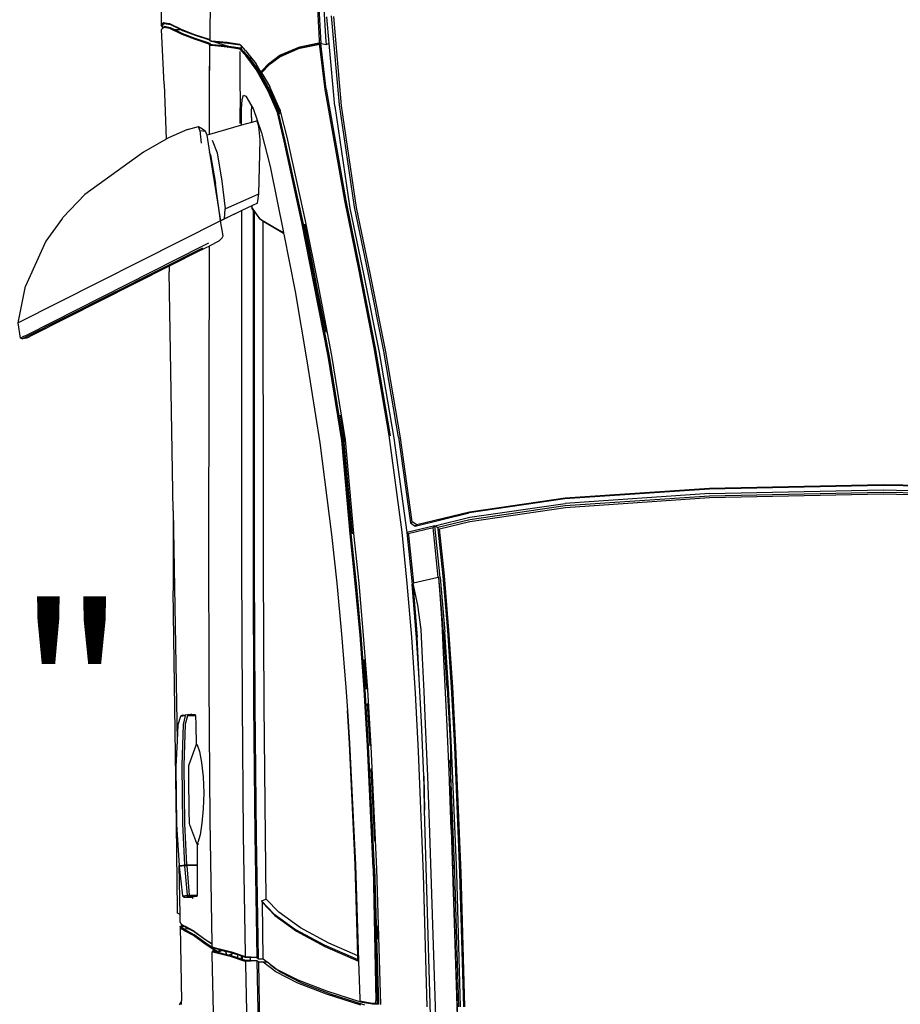
# Model space of a CAD drawing. Units: inches. Extents: x 0 to 4258, y 0 to 3769.
# Tile 10 of 30: x 3726 to 3761, y 3042 to 3082. Entities that reach past the tile are written whole.
import ezdxf

# ---------------------------------------------------------------- set-up
doc = ezdxf.new("R2010")
doc.units = ezdxf.units.IN
doc.header["$MEASUREMENT"] = 0
doc.layers.get('0').update_dxf_attribs({"color": 16})
doc.layers.add('A-ANNO-DIMS', color=250, linetype='Continuous', lineweight=18)
doc.layers.add('C-PKNG-VEHI', color=8, linetype='Continuous', lineweight=18)
doc.layers.add('Edges', color=250, linetype='Continuous')
doc.styles.get("Standard").update_dxf_attribs({"font": 'arial.ttf'})
doc.dimstyles.get("Standard").update_dxf_attribs({"dimtxt": 7, "dimasz": 0.18, "dimexe": 0.18, "dimexo": 0.0625, "dimgap": 0.09, "dimtad": 0, "dimtih": 1, "dimtoh": 1, "dimzin": 0, "dimdsep": 46, "dimlunit": 3, "dimtxsty": 'Standard', "dimcen": 0.09, "dimadec": 0, "dimazin": 0, "dimtfac": 1, "dimtofl": 0, "dimtmove": 0, "dimatfit": 3, "dimfxl": 1, "dimtolj": 1, "dimtzin": 0, "dimarcsym": 0})

# ---------------------------------------------------------------- blocks, each defined once
blk = doc.blocks.new('Nissan Qashqai pl')
at = {"layer": 'Edges'}
for p, q in [((9.2241, 12.1376), (9.2195, 11.9221)), ((9.2249, 12.1376), (9.2203, 11.9221)), ((9.2259, 11.9221), (9.2305, 12.1375)), ((9.2335, 12.1374), (9.2289, 11.9221)), ((9.2308, 11.9221), (9.2355, 12.1374)), ((9.2195, 11.9221), (9.2241, 11.7066)), ((9.2203, 11.9221), (9.2249, 11.7065)), ((9.2305, 11.7067), (9.2259, 11.9221)), ((9.2289, 11.9221), (9.2335, 11.7067)), ((9.2355, 11.7068), (9.2308, 11.9221)), ((9.2241, 11.7066), (9.2362, 11.5274)), ((9.2249, 11.7065), (9.2371, 11.5273)), ((9.2305, 11.7067), (9.2426, 11.5277)), ((9.2335, 11.7067), (9.2457, 11.5277)), ((9.2476, 11.5278), (9.2355, 11.7068)), ((9.2362, 11.5274), (9.2535, 11.4087)), ((9.2371, 11.5273), (9.2543, 11.4085)), ((9.2598, 11.4093), (9.2426, 11.5277)), ((9.2457, 11.5277), (9.2629, 11.4092)), ((9.2649, 11.4094), (9.2476, 11.5278)), ((9.2535, 11.4087), (9.2694, 11.3436)), ((9.2707, 11.3414), (9.2543, 11.4085)), ((9.2704, 11.3659), (9.2598, 11.4093)), ((9.2629, 11.4092), (9.2726, 11.3695)), ((9.2741, 11.3716), (9.2649, 11.4094)), ((9.8673, 11.4031), (9.701, 11.3983)), ((9.7011, 11.3963), (9.8673, 11.4012)), ((9.4706, 11.388), (9.4, 11.3832)), ((9.5443, 11.3919), (9.4706, 11.388)), ((9.4709, 11.3861), (9.5446, 11.39)), ((9.701, 11.3983), (9.5443, 11.3919)), ((9.5446, 11.39), (9.7011, 11.3963)), ((9.7014, 11.3929), (9.5454, 11.3866)), ((9.7014, 11.3906), (9.5695, 11.3853)), ((9.6472, 11.3861), (9.9278, 11.3949)), ((9.6714, 11.3874), (9.8565, 11.3931)), ((9.8673, 11.3977), (9.7014, 11.3929)), ((9.8673, 11.3954), (9.7014, 11.3906)), ((9.8565, 11.3931), (9.9794, 11.3967)), ((9.3326, 11.3776), (9.2741, 11.3716)), ((9.2746, 11.3697), (9.333, 11.3757)), ((9.4, 11.3832), (9.3326, 11.3776)), ((9.333, 11.3757), (9.4004, 11.3813)), ((9.4017, 11.3765), (9.3344, 11.3708)), ((9.3346, 11.3724), (9.4018, 11.378)), ((9.4276, 11.3767), (9.3918, 11.3747)), ((9.4004, 11.3813), (9.4709, 11.3861)), ((9.472, 11.3812), (9.4017, 11.3765)), ((9.472, 11.3828), (9.4018, 11.378)), ((9.4694, 11.3788), (9.4276, 11.3767)), ((9.5105, 11.3805), (9.4694, 11.3788)), ((9.5454, 11.3866), (9.472, 11.3828)), ((9.472, 11.3812), (9.5454, 11.3851)), ((9.5755, 11.3834), (9.5105, 11.3805)), ((9.5454, 11.3851), (9.5695, 11.3853)), ((9.5454, 11.3848), (9.5454, 11.3851)), ((9.5695, 11.3853), (9.5609, 11.3849)), ((9.5695, 11.3853), (9.5786, 11.3853)), ((9.6472, 11.3861), (9.5755, 11.3834)), ((9.5786, 11.3853), (9.6206, 11.3861)), ((9.6206, 11.3861), (9.6714, 11.3874)), ((9.3346, 11.3724), (9.2704, 11.3659)), ((9.2704, 11.3659), (9.2726, 11.3695)), ((9.2704, 11.3659), (9.2724, 11.3637)), ((9.2704, 11.3659), (9.2789, 11.331)), ((9.3346, 11.37), (9.2724, 11.3637)), ((9.2799, 11.3328), (9.2724, 11.3637)), ((9.2726, 11.3695), (9.2746, 11.3697)), ((9.3611, 11.3727), (9.3344, 11.3708)), ((9.3344, 11.3708), (9.3346, 11.37)), ((9.3346, 11.37), (9.3418, 11.3391)), ((9.3918, 11.3747), (9.3611, 11.3727)), ((9.6514, 11.3592), (9.9312, 11.3681)), ((9.4347, 11.3502), (9.4761, 11.3522)), ((9.4761, 11.3522), (9.5168, 11.3539)), ((9.5811, 11.3522), (9.514, 11.3492)), ((9.5168, 11.3539), (9.5812, 11.3568)), ((9.7029, 11.3516), (9.5503, 11.3455)), ((9.5811, 11.3522), (9.6231, 11.3531)), ((9.594, 11.3527), (9.5811, 11.3522)), ((9.5812, 11.3568), (9.6514, 11.3592)), ((9.6231, 11.3531), (9.594, 11.3527)), ((9.651, 11.3536), (9.6231, 11.3531)), ((9.9583, 11.363), (9.651, 11.3536)), ((9.8673, 11.3563), (9.7029, 11.3516)), ((9.2694, 11.3436), (9.2656, 11.3376)), ((9.2669, 11.3354), (9.2707, 11.3414)), ((9.2694, 11.3436), (9.2707, 11.3414)), ((9.2819, 11.333), (9.3418, 11.3391)), ((9.3418, 11.3391), (9.342, 11.3383)), ((9.342, 11.3383), (9.3687, 11.3441)), ((9.342, 11.3383), (9.4087, 11.3438)), ((9.4093, 11.3431), (9.3427, 11.3375)), ((9.3687, 11.3441), (9.3992, 11.3482)), ((9.3992, 11.3482), (9.4347, 11.3502)), ((9.4605, 11.3465), (9.4087, 11.3438)), ((9.4782, 11.3418), (9.4088, 11.3371)), ((9.4605, 11.3465), (9.4093, 11.3431)), ((9.514, 11.3492), (9.4605, 11.3465)), ((9.5503, 11.3455), (9.4782, 11.3418)), ((9.1605, 11.3208), (9.2669, 11.3354)), ((9.2656, 11.3376), (9.1612, 11.3233)), ((9.1617, 11.315), (9.2789, 11.331)), ((9.2669, 11.3354), (9.2656, 11.3376)), ((9.3422, 11.3316), (9.2783, 11.3251)), ((9.2789, 11.331), (9.3427, 11.3375)), ((9.2789, 11.331), (9.2799, 11.3327)), ((9.2799, 11.3328), (9.2819, 11.333)), ((9.2799, 11.3327), (9.2799, 11.3328)), ((9.2799, 11.3327), (9.2811, 11.3325)), ((9.4088, 11.3371), (9.3422, 11.3316)), ((9.1605, 11.3208), (9.0538, 11.3023)), ((9.1612, 11.3233), (9.0546, 11.3048)), ((9.0552, 11.2965), (9.1617, 11.315)), ((9.2783, 11.3251), (9.1584, 11.3091)), ((9.0538, 11.3023), (8.9583, 11.2833)), ((9.0546, 11.3048), (8.9591, 11.2859)), ((9.1584, 11.3091), (9.0495, 11.2906)), ((9.0497, 11.2918), (9.1586, 11.3104)), ((9.0495, 11.2906), (8.9521, 11.2715)), ((8.9522, 11.2728), (9.0497, 11.2918)), ((8.9598, 11.2775), (9.0552, 11.2965)), ((9.6954, 11.2907), (9.5438, 11.2836)), ((9.5443, 11.2863), (9.696, 11.2932)), ((9.5717, 11.2865), (9.6618, 11.2907)), ((9.6953, 11.2892), (9.863, 11.2944)), ((9.6953, 11.2892), (9.8598, 11.2925)), ((9.6954, 11.2907), (9.8641, 11.2959)), ((9.696, 11.2932), (9.8644, 11.2982)), ((9.7669, 11.2945), (9.7832, 11.2951)), ((9.8629, 11.2925), (9.8598, 11.2925)), ((9.8626, 11.2878), (9.8627, 11.2909)), ((9.8627, 11.2909), (9.8629, 11.2925)), ((9.8627, 11.2909), (9.8637, 11.291)), ((9.8629, 11.2925), (9.863, 11.2944)), ((9.8641, 11.2959), (9.863, 11.2944)), ((9.8635, 11.2886), (9.8637, 11.291)), ((9.8637, 11.291), (9.8638, 11.2934)), ((9.8637, 11.291), (9.8643, 11.291)), ((9.8638, 11.2934), (9.8641, 11.2959)), ((8.9583, 11.2833), (8.8745, 11.266)), ((8.9591, 11.2859), (8.8754, 11.2687)), ((8.8761, 11.2602), (8.9598, 11.2775)), ((9.4735, 11.2779), (9.4062, 11.2729)), ((9.4736, 11.2793), (9.4063, 11.2743)), ((9.4064, 11.277), (9.4739, 11.282)), ((9.4727, 11.2808), (9.4362, 11.278)), ((9.4727, 11.2808), (9.4732, 11.2808)), ((9.5437, 11.2822), (9.4735, 11.2779)), ((9.5438, 11.2836), (9.4736, 11.2793)), ((9.4739, 11.282), (9.5443, 11.2863)), ((9.491, 11.2819), (9.5434, 11.2852)), ((9.6953, 11.2892), (9.5437, 11.2822)), ((9.8652, 11.2788), (9.8516, 11.2363)), ((9.8605, 11.2746), (9.8626, 11.2878)), ((9.8615, 11.2754), (9.8635, 11.2886)), ((8.8745, 11.266), (8.7481, 11.2473)), ((8.8754, 11.2687), (8.7491, 11.2501)), ((8.8666, 11.2554), (8.9522, 11.2728)), ((8.9521, 11.2715), (8.8666, 11.2541)), ((9.2801, 11.2648), (9.3418, 11.2713)), ((9.3418, 11.2671), (9.2803, 11.2606)), ((9.3419, 11.2685), (9.2804, 11.262)), ((9.3418, 11.2713), (9.4064, 11.277)), ((9.4062, 11.2729), (9.3418, 11.2671)), ((9.4063, 11.2743), (9.3419, 11.2685)), ((9.5403, 11.26), (9.6913, 11.2674)), ((9.6912, 11.2667), (9.5404, 11.2598)), ((9.8039, 11.27), (9.6912, 11.2667)), ((9.6913, 11.2674), (9.8099, 11.2711)), ((9.8039, 11.27), (9.7884, 11.2343)), ((9.7905, 11.2283), (9.8087, 11.2702)), ((9.7925, 11.2294), (9.8107, 11.2711)), ((9.8087, 11.2702), (9.8039, 11.27)), ((9.8099, 11.2711), (9.8087, 11.2702)), ((9.8099, 11.2711), (9.8107, 11.2711)), ((9.8107, 11.2711), (9.8573, 11.2726)), ((9.8475, 11.2312), (9.8611, 11.2734)), ((9.8652, 11.2738), (9.8516, 11.2313)), ((9.8573, 11.2726), (9.8603, 11.2727)), ((9.8603, 11.2727), (9.8605, 11.2746)), ((9.8611, 11.2734), (9.8603, 11.2727)), ((9.8612, 11.2735), (9.8611, 11.2734)), ((9.8612, 11.2735), (9.8615, 11.2754)), ((8.7287, 11.2307), (8.8666, 11.2554)), ((8.8666, 11.2541), (8.7292, 11.2295)), ((8.7496, 11.2416), (8.8761, 11.2602)), ((9.0591, 11.2377), (9.1639, 11.2546)), ((9.133, 11.2481), (9.1647, 11.2532)), ((9.1639, 11.2546), (9.2801, 11.2648)), ((9.2803, 11.2606), (9.1644, 11.2503)), ((9.2804, 11.262), (9.1645, 11.2518)), ((9.1647, 11.2532), (9.1668, 11.2533)), ((9.2804, 11.2635), (9.1668, 11.2533)), ((9.4048, 11.2501), (9.471, 11.2554)), ((9.471, 11.2554), (9.4997, 11.2573)), ((9.4997, 11.2573), (9.5403, 11.26)), ((9.5404, 11.2598), (9.4997, 11.2573)), ((8.7481, 11.2473), (8.6375, 11.2376)), ((8.7491, 11.2501), (8.6386, 11.2404)), ((8.7496, 11.2416), (8.6721, 11.2348)), ((9.1644, 11.2503), (9.06, 11.2335)), ((9.1645, 11.2518), (9.0601, 11.235)), ((9.2814, 11.2377), (9.3416, 11.2442)), ((9.3416, 11.2442), (9.4048, 11.2501)), ((8.6699, 11.231), (8.622, 11.228)), ((8.6721, 11.2348), (8.6387, 11.2319)), ((8.6721, 11.2312), (8.6699, 11.231)), ((8.6721, 11.2348), (8.6733, 11.2313)), ((8.6721, 11.2312), (8.6721, 11.2318)), ((8.6721, 11.2241), (8.6733, 11.2313)), ((8.6733, 11.2313), (8.6721, 11.2312)), ((8.7287, 11.2307), (8.6721, 11.2241)), ((8.7292, 11.2295), (8.6753, 11.2232)), ((9.0601, 11.235), (8.8941, 11.2023)), ((8.9679, 11.2201), (9.0591, 11.2377)), ((9.06, 11.2335), (8.9696, 11.2157)), ((8.9708, 11.2185), (9.03, 11.2304)), ((9.1676, 11.2229), (9.2814, 11.2377)), ((9.7884, 11.2343), (9.7692, 11.1989)), ((9.7733, 11.194), (9.7925, 11.2294)), ((9.8338, 11.1956), (9.8475, 11.2312)), ((9.8516, 11.2363), (9.8378, 11.2007)), ((9.8516, 11.2313), (9.8378, 11.1957)), ((8.6683, 11.2226), (8.6197, 11.2201)), ((8.6203, 11.2213), (8.6721, 11.2241)), ((8.671, 11.2227), (8.6683, 11.2226)), ((8.6721, 11.2241), (8.671, 11.2227)), ((8.6716, 11.2199), (8.671, 11.2227)), ((8.6759, 11.1982), (8.6716, 11.2199)), ((8.6721, 11.2241), (8.6727, 11.2229)), ((8.6772, 11.1988), (8.6721, 11.2241)), ((8.6753, 11.2232), (8.6727, 11.2229)), ((8.6777, 11.1984), (8.6727, 11.2229)), ((8.8918, 11.205), (8.9679, 11.2201)), ((8.9318, 11.211), (8.9704, 11.2185)), ((8.9704, 11.2185), (8.9708, 11.2185)), ((9.0656, 11.207), (9.1676, 11.2229)), ((9.7713, 11.1929), (9.7905, 11.2283)), ((8.7881, 11.1821), (8.8918, 11.205)), ((8.9696, 11.2157), (8.8942, 11.2009)), ((8.8961, 11.204), (8.9318, 11.211)), ((8.9797, 11.1924), (9.0656, 11.207)), ((8.6864, 11.1736), (8.6759, 11.1982)), ((8.6875, 11.1744), (8.6772, 11.1988)), ((8.6777, 11.1984), (8.6883, 11.1737)), ((8.8941, 11.2023), (8.7925, 11.1802)), ((8.8942, 11.2009), (8.7931, 11.1789)), ((8.9087, 11.1783), (8.9797, 11.1924)), ((9.7692, 11.1989), (9.7499, 11.1721)), ((9.7519, 11.1661), (9.7713, 11.1929)), ((9.754, 11.1672), (9.7733, 11.194)), ((9.8201, 11.1685), (9.8338, 11.1956)), ((9.8378, 11.2007), (9.8241, 11.1736)), ((9.8378, 11.1957), (9.8241, 11.1686)), ((8.7575, 11.1744), (8.7881, 11.1821)), ((8.7925, 11.1802), (8.7591, 11.1723)), ((8.697, 11.1592), (8.6864, 11.1736)), ((8.6979, 11.1603), (8.6875, 11.1744)), ((8.6883, 11.1737), (8.6987, 11.1597)), ((8.7508, 11.1722), (8.7257, 11.1609)), ((8.7529, 11.17), (8.7302, 11.1602)), ((8.7574, 11.1704), (8.7312, 11.1591)), ((8.7346, 11.1636), (8.7577, 11.1732)), ((8.7346, 11.1636), (8.7491, 11.1703)), ((8.7491, 11.1703), (8.7576, 11.1743)), ((8.7508, 11.1722), (8.7491, 11.1703)), ((8.7532, 11.1733), (8.7508, 11.1722)), ((8.7529, 11.17), (8.7577, 11.1732)), ((8.757, 11.1718), (8.7529, 11.17)), ((8.7532, 11.1733), (8.7575, 11.1744)), ((8.7587, 11.1722), (8.757, 11.1718)), ((8.7931, 11.1789), (8.7574, 11.1704)), ((8.7575, 11.1744), (8.7576, 11.1743)), ((8.7576, 11.1743), (8.7582, 11.1734)), ((8.7577, 11.1732), (8.7582, 11.1734)), ((8.7582, 11.1734), (8.759, 11.1725)), ((8.759, 11.1725), (8.7587, 11.1722)), ((8.7591, 11.1723), (8.7587, 11.1722)), ((8.759, 11.1725), (8.7591, 11.1723)), ((8.8245, 11.1613), (8.9063, 11.1779)), ((8.8893, 11.1486), (8.9021, 11.1697)), ((8.9041, 11.1717), (8.8927, 11.1528)), ((8.9021, 11.1697), (8.9063, 11.1779)), ((8.9075, 11.1781), (8.9041, 11.1717)), ((8.9063, 11.1779), (8.9075, 11.1781)), ((8.9075, 11.1781), (8.9087, 11.1783)), ((9.7499, 11.1721), (9.7337, 11.1566)), ((9.8241, 11.1686), (9.8119, 11.1529)), ((9.8241, 11.1736), (9.8147, 11.1616)), ((9.8147, 11.1616), (9.8201, 11.1685)), ((8.7055, 11.1514), (8.697, 11.1592)), ((8.6987, 11.1596), (8.6979, 11.1603)), ((8.6987, 11.1597), (8.6988, 11.1596)), ((8.6987, 11.1596), (8.6988, 11.1596)), ((8.6996, 11.1588), (8.6987, 11.1596)), ((8.6988, 11.1596), (8.6996, 11.1588)), ((8.6996, 11.1588), (8.6996, 11.1588)), ((8.7062, 11.1527), (8.6996, 11.1588)), ((8.6996, 11.1588), (8.7062, 11.1527)), ((8.7302, 11.1602), (8.7032, 11.145)), ((8.7312, 11.1591), (8.7042, 11.144)), ((8.7075, 11.1487), (8.7346, 11.1636)), ((8.7108, 11.1523), (8.7257, 11.1609)), ((8.7108, 11.1523), (8.7248, 11.1605)), ((8.7248, 11.1605), (8.7257, 11.1609)), ((8.7828, 11.1508), (8.8245, 11.1613)), ((9.6552, 11.1554), (9.4936, 11.1538)), ((9.7337, 11.1566), (9.6552, 11.1554)), ((9.7357, 11.1507), (9.7337, 11.1566)), ((9.7357, 11.1507), (9.7519, 11.1661)), ((9.7378, 11.1517), (9.754, 11.1672)), ((9.8078, 11.1528), (9.8119, 11.1579)), ((9.8147, 11.1616), (9.8119, 11.1579)), ((9.8119, 11.1579), (9.8119, 11.1529)), ((9.8147, 11.1616), (9.8147, 11.1616)), ((8.7042, 11.144), (8.687, 11.131)), ((8.6884, 11.1371), (8.6973, 11.144)), ((8.6917, 11.1371), (8.7075, 11.1487)), ((8.7032, 11.145), (8.6927, 11.1371)), ((8.6973, 11.144), (8.698, 11.1446)), ((8.698, 11.1446), (8.6981, 11.1446)), ((8.7071, 11.15), (8.6981, 11.1446)), ((8.707, 11.15), (8.7055, 11.1514)), ((8.7067, 11.1522), (8.7062, 11.1527)), ((8.7083, 11.1508), (8.7067, 11.1522)), ((8.707, 11.15), (8.7083, 11.1508)), ((8.7071, 11.15), (8.707, 11.15)), ((8.707, 11.15), (8.707, 11.15)), ((8.7083, 11.1508), (8.7071, 11.15)), ((8.7083, 11.1507), (8.7102, 11.1519)), ((8.7083, 11.1508), (8.7083, 11.1507)), ((8.7102, 11.1519), (8.7108, 11.1523)), ((8.7524, 11.1401), (8.7828, 11.1508)), ((8.7748, 11.1475), (8.7678, 11.1453)), ((8.7678, 11.1453), (8.7698, 11.1385)), ((8.7916, 11.1488), (8.7748, 11.1475)), ((8.8259, 11.1483), (8.7916, 11.1488)), ((8.8585, 11.1473), (8.8259, 11.1483)), ((8.87, 11.1455), (8.8585, 11.1473)), ((8.8771, 11.1054), (8.8585, 11.1473)), ((8.87, 11.1455), (8.8734, 11.1385)), ((8.8893, 11.1486), (8.8751, 11.1387)), ((8.881, 11.1418), (8.8893, 11.1486)), ((8.8913, 11.1506), (8.8893, 11.1486)), ((8.8927, 11.1528), (8.8913, 11.1506)), ((9.3225, 11.1531), (8.8927, 11.1528)), ((9.4936, 11.1538), (9.3225, 11.1531)), ((9.6552, 11.1445), (9.4936, 11.1428)), ((9.654, 11.1423), (9.8061, 11.1447)), ((9.8078, 11.1471), (9.6552, 11.1445)), ((9.7357, 11.1507), (9.7378, 11.1517)), ((9.8078, 11.1528), (9.7378, 11.1517)), ((9.8061, 11.1447), (9.8051, 11.1309)), ((9.8058, 11.1369), (9.8061, 11.1447)), ((9.8061, 11.1447), (9.8078, 11.1471)), ((9.8078, 11.1471), (9.8078, 11.1528)), ((9.8101, 11.1449), (9.8098, 11.1369)), ((9.8101, 11.1449), (9.9411, 11.1475)), ((9.8119, 11.1472), (9.8101, 11.1449)), ((9.8101, 11.1449), (9.8112, 11.1311)), ((9.8119, 11.1529), (9.8119, 11.1472)), ((9.9393, 11.1497), (9.8119, 11.1472)), ((8.6805, 11.1309), (8.6746, 11.1253)), ((8.687, 11.131), (8.6788, 11.1237)), ((8.6805, 11.1309), (8.6884, 11.1371)), ((8.6859, 11.132), (8.6817, 11.1282)), ((8.6818, 11.1288), (8.6902, 11.136)), ((8.6927, 11.1371), (8.6859, 11.132)), ((8.6884, 11.1371), (8.6917, 11.1371)), ((8.6902, 11.136), (8.6917, 11.1371)), ((8.6923, 11.1371), (8.6927, 11.1371)), ((8.7361, 11.1283), (8.7373, 11.1314)), ((8.7373, 11.1314), (8.7492, 11.1383)), ((8.7492, 11.1383), (8.7524, 11.1401)), ((8.7492, 11.1383), (8.7572, 11.1379)), ((8.7572, 11.1379), (8.7698, 11.1383)), ((8.7698, 11.1385), (8.7583, 11.1382)), ((8.7698, 11.1385), (8.7698, 11.1383)), ((8.7698, 11.1383), (8.7733, 11.126)), ((8.8734, 11.1385), (8.8793, 11.1261)), ((8.8734, 11.1385), (8.8768, 11.1385)), ((8.8751, 11.1387), (8.8768, 11.1385)), ((8.8768, 11.1385), (8.879, 11.1402)), ((8.879, 11.1402), (8.881, 11.1418)), ((8.879, 11.1402), (9.3198, 11.1403)), ((9.3225, 11.1421), (8.881, 11.1418)), ((9.3198, 11.1403), (9.4922, 11.1409)), ((9.4936, 11.1428), (9.3225, 11.1421)), ((9.4922, 11.1409), (9.654, 11.1423)), ((9.802, 11.1309), (9.6538, 11.1284)), ((9.8051, 11.1309), (9.802, 11.1309)), ((9.8044, 11.129), (9.8051, 11.1309)), ((9.8055, 11.1298), (9.8058, 11.1369)), ((9.8098, 11.1369), (9.8058, 11.1369)), ((9.8098, 11.1369), (9.8096, 11.13)), ((9.8112, 11.1311), (9.8106, 11.1292)), ((9.8143, 11.1312), (9.8112, 11.1311)), ((9.9414, 11.1341), (9.8143, 11.1312)), ((8.6703, 11.1081), (8.6727, 11.1235)), ((8.6714, 11.1088), (8.6737, 11.1245)), ((8.6727, 11.1235), (8.6737, 11.1245)), ((8.6737, 11.1245), (8.6746, 11.1253)), ((8.6746, 11.1253), (8.6785, 11.1253)), ((8.6777, 11.1246), (8.6755, 11.1099)), ((8.6788, 11.1237), (8.6764, 11.1083)), ((8.6785, 11.1253), (8.6777, 11.1246)), ((8.6815, 11.128), (8.6785, 11.1253)), ((8.6815, 11.128), (8.6818, 11.1288)), ((8.6817, 11.1282), (8.6815, 11.128)), ((8.6817, 11.1282), (8.6818, 11.1288)), ((8.6818, 11.1238), (8.7026, 11.1238)), ((8.7026, 11.1238), (8.7026, 11.1239)), ((8.7026, 11.1238), (8.7072, 11.1239)), ((8.7072, 11.1239), (8.7072, 11.1239)), ((8.7072, 11.1239), (8.7273, 11.1239)), ((8.7273, 11.1239), (8.7273, 11.124)), ((8.7273, 11.1239), (8.7354, 11.124)), ((8.7354, 11.1241), (8.7354, 11.124)), ((8.7354, 11.124), (8.742, 11.124)), ((8.7415, 11.1265), (8.7361, 11.1283)), ((8.7534, 11.1257), (8.7415, 11.1265)), ((8.742, 11.1241), (8.742, 11.124)), ((8.742, 11.124), (8.742, 11.1241)), ((8.742, 11.124), (8.742, 11.124)), ((8.742, 11.124), (8.7426, 11.124)), ((8.7426, 11.1241), (8.7426, 11.124)), ((8.7426, 11.124), (8.7433, 11.124)), ((8.7433, 11.1241), (8.7433, 11.124)), ((8.7433, 11.124), (8.7711, 11.1241)), ((8.7711, 11.1241), (8.7516, 11.1241)), ((8.7718, 11.126), (8.7534, 11.1257)), ((8.7733, 11.126), (8.7718, 11.126)), ((8.7733, 11.126), (8.7849, 11.0859)), ((9.3194, 11.1262), (8.8793, 11.1261)), ((8.8793, 11.1261), (8.8815, 11.1214)), ((8.8815, 11.1214), (8.892, 11.0998)), ((8.8815, 11.1214), (8.8895, 11.1048)), ((9.4919, 11.1269), (9.3194, 11.1262)), ((9.6538, 11.1284), (9.4919, 11.1269)), ((9.7992, 11.1133), (9.8044, 11.129)), ((9.803, 11.1212), (9.8014, 11.1176)), ((9.8014, 11.1176), (9.8026, 11.1212)), ((9.8026, 11.1212), (9.8041, 11.1256)), ((9.803, 11.1212), (9.8026, 11.1212)), ((9.8067, 11.1213), (9.803, 11.1212)), ((9.8041, 11.1256), (9.8045, 11.1268)), ((9.8041, 11.1256), (9.8081, 11.1256)), ((9.8067, 11.1213), (9.8044, 11.1142)), ((9.8045, 11.1268), (9.8046, 11.1271)), ((9.8045, 11.1268), (9.8085, 11.1268)), ((9.8046, 11.1271), (9.8055, 11.1298)), ((9.8086, 11.1271), (9.8046, 11.1271)), ((9.8106, 11.1292), (9.8054, 11.1135)), ((9.8081, 11.1256), (9.8067, 11.1213)), ((9.8085, 11.1268), (9.8081, 11.1256)), ((9.8086, 11.1271), (9.8085, 11.1268)), ((9.8096, 11.13), (9.8086, 11.1271)), ((8.6684, 11.0892), (8.6703, 11.1081)), ((8.6697, 11.0922), (8.6714, 11.1088)), ((8.6698, 11.0925), (8.6755, 11.1099)), ((8.6754, 11.1089), (8.6735, 11.0898)), ((8.6764, 11.1082), (8.6744, 11.0891)), ((8.6755, 11.1099), (8.6754, 11.1089)), ((8.6764, 11.1082), (8.6764, 11.1083)), ((9.7937, 11.0918), (9.7992, 11.1133)), ((9.7978, 11.1044), (9.7987, 11.108)), ((9.7987, 11.108), (9.8002, 11.1141)), ((9.7992, 11.1065), (9.7987, 11.108)), ((9.7992, 11.1065), (9.7987, 11.1053)), ((9.8027, 11.1078), (9.7992, 11.1065)), ((9.8054, 11.1135), (9.7999, 11.0919)), ((9.8002, 11.1141), (9.8008, 11.1157)), ((9.8027, 11.1078), (9.8003, 11.0983)), ((9.8008, 11.1157), (9.8014, 11.1176)), ((9.8014, 11.1139), (9.8008, 11.1157)), ((9.8043, 11.1139), (9.8014, 11.1139)), ((9.8031, 11.1093), (9.8014, 11.1139)), ((9.8031, 11.1093), (9.8027, 11.1078)), ((9.8043, 11.1139), (9.8031, 11.1093)), ((9.8044, 11.1142), (9.8043, 11.1139)), ((8.7917, 11.0895), (8.8075, 11.0955)), ((8.807, 11.0862), (8.8918, 11.0997)), ((8.8075, 11.0955), (8.8429, 11.1016)), ((8.8429, 11.1016), (8.8771, 11.1054)), ((8.8918, 11.0997), (8.8455, 11.0936)), ((8.8895, 11.1048), (8.8771, 11.1054)), ((8.8908, 11.1021), (8.8895, 11.1048)), ((8.8906, 11.1024), (8.8895, 11.1048)), ((8.8906, 11.1024), (8.8911, 11.1013)), ((8.892, 11.0998), (8.8908, 11.1021)), ((8.8911, 11.1013), (8.8919, 11.0997)), ((8.8911, 11.1013), (8.8919, 11.0998)), ((8.8919, 11.0997), (8.8911, 11.1013)), ((8.8919, 11.0997), (8.8918, 11.0997)), ((8.8918, 11.0997), (9.0186, 10.8486)), ((8.892, 11.0998), (8.8919, 11.0998)), ((8.8919, 11.0998), (8.8919, 11.0997)), ((8.8919, 11.0997), (8.8919, 11.0997)), ((8.9106, 11.1029), (8.892, 11.0998)), ((8.892, 11.0998), (8.892, 11.0998)), ((8.9131, 11.102), (8.9106, 11.1029)), ((8.9171, 11.0978), (8.9131, 11.102)), ((8.9171, 11.0978), (8.917, 11.0974)), ((8.9171, 11.0978), (8.9233, 11.0855)), ((9.7964, 11.0988), (9.7943, 11.0907)), ((9.7992, 11.0966), (9.7963, 11.0918)), ((9.7964, 11.0988), (9.7973, 11.1023)), ((9.7964, 11.0988), (9.7992, 11.0966)), ((9.7964, 11.0917), (9.7996, 11.0966)), ((9.7973, 11.1023), (9.7977, 11.1042)), ((9.7977, 11.1033), (9.7973, 11.1023)), ((9.7973, 11.1023), (9.7977, 11.1011)), ((9.7987, 11.1053), (9.7977, 11.1033)), ((9.7977, 11.1042), (9.7978, 11.1044)), ((9.7977, 11.1042), (9.7977, 11.1033)), ((9.7977, 11.1011), (9.7977, 11.0998)), ((9.7977, 11.1011), (9.7985, 11.099)), ((9.7977, 11.0998), (9.7985, 11.099)), ((9.7987, 11.1053), (9.7978, 11.1044)), ((9.7985, 11.099), (9.7989, 11.098)), ((9.7998, 11.0964), (9.7988, 11.0925)), ((9.7989, 11.098), (9.7998, 11.0976)), ((9.7998, 11.0976), (9.7992, 11.0966)), ((9.8002, 11.098), (9.7996, 11.0966)), ((9.8001, 11.0974), (9.7996, 11.0966)), ((9.7996, 11.0966), (9.7998, 11.0964)), ((9.8003, 11.0983), (9.7998, 11.0976)), ((9.8001, 11.0974), (9.7998, 11.0964)), ((9.8002, 11.098), (9.8001, 11.0974)), ((9.8003, 11.0983), (9.8002, 11.098)), ((8.5326, 11.0874), (8.6675, 11.0866)), ((8.6606, 11.0674), (8.6667, 11.0857)), ((8.6616, 11.0683), (8.6675, 11.0862)), ((8.6718, 11.0868), (8.6657, 11.0684)), ((8.6667, 11.0857), (8.6675, 11.0862)), ((8.6728, 11.0858), (8.6667, 11.0675)), ((8.6674, 11.0864), (8.6675, 11.0865)), ((8.6675, 11.0865), (8.6675, 11.0866)), ((8.6676, 11.0866), (8.6675, 11.0866)), ((8.6675, 11.0862), (8.6679, 11.0864)), ((8.6676, 11.0864), (8.6677, 11.0866)), ((8.6677, 11.0866), (8.6676, 11.0866)), ((8.6682, 11.0866), (8.6677, 11.0866)), ((8.6679, 11.0864), (8.6682, 11.0866)), ((8.6682, 11.087), (8.6684, 11.0888)), ((8.6692, 11.0876), (8.6682, 11.0866)), ((8.6682, 11.087), (8.6692, 11.0876)), ((8.6682, 11.0866), (8.6682, 11.087)), ((8.6684, 11.0888), (8.6684, 11.0892)), ((8.6684, 11.0888), (8.6685, 11.089)), ((8.6692, 11.0876), (8.6697, 11.0922)), ((8.6697, 11.0922), (8.6698, 11.0925)), ((8.6729, 11.0874), (8.6718, 11.0868)), ((8.674, 11.0864), (8.6728, 11.0858)), ((8.6733, 11.0875), (8.6729, 11.0874)), ((8.6735, 11.0898), (8.6733, 11.0875)), ((8.6742, 11.0866), (8.674, 11.0864)), ((8.6744, 11.0891), (8.6742, 11.0866)), ((8.6744, 11.0866), (8.6742, 11.0866)), ((8.6742, 11.0858), (8.6743, 11.086)), ((8.6744, 11.0864), (8.6744, 11.0866)), ((8.6773, 11.0865), (8.6744, 11.0866)), ((8.6791, 11.0864), (8.677, 11.0864)), ((8.6791, 11.0865), (8.6773, 11.0865)), ((8.6791, 11.0865), (8.6791, 11.0864)), ((8.6878, 11.0864), (8.6791, 11.0865)), ((8.7205, 11.0863), (8.6791, 11.0864)), ((8.6878, 11.0864), (8.6791, 11.0864)), ((8.6878, 11.0865), (8.6878, 11.0864)), ((8.6911, 11.0864), (8.6878, 11.0864)), ((8.7205, 11.0863), (8.6911, 11.0864)), ((8.7849, 11.0859), (8.7205, 11.0863)), ((8.7849, 11.0827), (8.7807, 11.0812)), ((8.7849, 11.0859), (8.7856, 11.0834)), ((8.7849, 11.0827), (8.7858, 11.0828)), ((8.7858, 11.0828), (8.7856, 11.0834)), ((8.7858, 11.0828), (8.807, 11.0862)), ((8.8102, 11.0874), (8.807, 11.0862)), ((8.8102, 11.0874), (8.8455, 11.0936)), ((8.9232, 11.0779), (8.9194, 11.0854)), ((8.9233, 11.0855), (9.2886, 11.0848)), ((8.925, 11.0821), (8.9233, 11.0855)), ((8.928, 11.0762), (8.925, 11.0821)), ((9.2886, 11.0848), (9.4673, 11.0852)), ((9.4673, 11.0852), (9.6358, 11.0866)), ((9.6358, 11.0866), (9.7887, 11.0889)), ((9.7832, 11.0805), (9.7887, 11.0889)), ((9.7842, 11.0814), (9.7891, 11.0889)), ((9.7933, 11.0892), (9.7883, 11.0815)), ((9.7887, 11.0889), (9.7891, 11.0889)), ((9.7891, 11.0889), (9.79, 11.0889)), ((9.7965, 11.0915), (9.7894, 11.0806)), ((9.79, 11.0889), (9.7931, 11.089)), ((9.7931, 11.089), (9.7934, 11.0906)), ((9.7931, 11.089), (9.7933, 11.0892)), ((9.7933, 11.0892), (9.7941, 11.0901)), ((9.7934, 11.0906), (9.7937, 11.0918)), ((9.7934, 11.0906), (9.7938, 11.0904)), ((9.7941, 11.0901), (9.7943, 11.0907)), ((9.7955, 11.0925), (9.7943, 11.0907)), ((9.7963, 11.0918), (9.7955, 11.0925)), ((9.7963, 11.0918), (9.7963, 11.0918)), ((9.7964, 11.0917), (9.7963, 11.0918)), ((9.7964, 11.0917), (9.7964, 11.0917)), ((9.7967, 11.0915), (9.7964, 11.0917)), ((9.7965, 11.0915), (9.7967, 11.0915)), ((9.7983, 11.0901), (9.7965, 11.0915)), ((9.7967, 11.0915), (9.7986, 11.0916)), ((9.7977, 11.0907), (9.7967, 11.0915)), ((9.7982, 11.0902), (9.7977, 11.0907)), ((9.7986, 11.0916), (9.7982, 11.0902)), ((9.7983, 11.0901), (9.7982, 11.0902)), ((9.7986, 11.0898), (9.7983, 11.0901)), ((9.7988, 11.0925), (9.7986, 11.0916)), ((9.7986, 11.0898), (9.7993, 11.0891)), ((9.7999, 11.0919), (9.7993, 11.0891)), ((9.7993, 11.0891), (9.8024, 11.0892)), ((9.8024, 11.0892), (9.9426, 11.0923)), ((8.7751, 11.0723), (8.7779, 11.0773)), ((8.7798, 11.0739), (8.7751, 11.0723)), ((8.7785, 11.0587), (8.7751, 11.0723)), ((8.7779, 11.0773), (8.7807, 11.0812)), ((8.7798, 11.0739), (8.7807, 11.0812)), ((8.7798, 11.0739), (8.7954, 11.0758)), ((9.0333, 10.8597), (8.9232, 11.0779)), ((9.0386, 10.8534), (8.9254, 11.0778)), ((8.928, 11.0762), (8.9483, 11.0359)), ((9.5422, 11.0706), (9.5422, 11.0716)), ((9.5422, 11.0706), (9.5424, 11.0707)), ((9.5423, 11.0696), (9.5422, 11.0706)), ((9.5424, 11.0707), (9.5503, 11.0736)), ((9.5426, 11.0695), (9.5424, 11.0707)), ((9.5503, 11.0736), (9.5641, 11.076)), ((9.5641, 11.076), (9.5818, 11.0782)), ((9.5818, 11.0782), (9.6016, 11.0791)), ((9.6016, 11.0791), (9.6215, 11.0782)), ((9.6215, 11.0782), (9.6395, 11.0766)), ((9.6395, 11.0766), (9.654, 11.0744)), ((9.6645, 11.0705), (9.6413, 11.0616)), ((9.654, 11.0744), (9.6633, 11.0715)), ((9.6633, 11.0715), (9.6645, 11.0705)), ((9.6655, 11.0708), (9.6645, 11.0705)), ((9.6655, 11.0728), (9.6655, 11.0708)), ((9.6655, 11.0708), (9.6911, 11.0709)), ((9.6911, 11.0709), (9.692, 11.0709)), ((9.6911, 11.0645), (9.6911, 11.0709)), ((9.692, 11.0709), (9.692, 11.0645)), ((9.692, 11.0709), (9.7287, 11.0708)), ((9.7287, 11.0708), (9.7305, 11.0704)), ((9.7288, 11.0609), (9.7287, 11.0708)), ((9.7305, 11.0704), (9.7313, 11.0644)), ((9.7305, 11.0704), (9.7306, 11.0607)), ((9.7728, 11.066), (9.7832, 11.0805)), ((9.7738, 11.067), (9.7842, 11.0814)), ((9.7883, 11.0815), (9.7778, 11.0671)), ((9.7894, 11.0806), (9.7788, 11.0661)), ((8.6546, 11.0516), (8.6606, 11.0674)), ((8.6556, 11.0524), (8.6616, 11.0683)), ((8.6657, 11.0684), (8.6598, 11.0529)), ((8.6667, 11.0675), (8.6608, 11.0521)), ((8.7785, 11.0587), (8.7891, 11.0353)), ((9.5037, 11.0635), (9.5045, 11.0628)), ((9.5044, 11.0586), (9.5045, 11.0628)), ((9.5052, 11.0524), (9.5044, 11.0586)), ((9.5045, 11.0683), (9.5063, 11.0687)), ((9.5045, 11.0628), (9.5045, 11.0683)), ((9.5063, 11.0687), (9.5061, 11.0586)), ((9.5061, 11.0586), (9.5167, 11.0559)), ((9.5063, 11.0687), (9.5168, 11.0691)), ((9.5168, 11.0691), (9.5423, 11.0696)), ((9.5426, 11.0695), (9.5423, 11.0696)), ((9.5667, 11.0609), (9.5426, 11.0695)), ((9.5678, 11.0604), (9.5667, 11.0609)), ((9.5846, 11.0606), (9.5678, 11.0604)), ((9.6236, 11.0609), (9.5846, 11.0606)), ((9.64, 11.0611), (9.6236, 11.0609)), ((9.6413, 11.0616), (9.64, 11.0611)), ((9.64, 11.0549), (9.6912, 11.0577)), ((9.6912, 11.0631), (9.6911, 11.0645)), ((9.692, 11.0631), (9.6912, 11.0631)), ((9.6912, 11.0577), (9.6912, 11.0631)), ((9.6913, 11.0556), (9.6912, 11.0577)), ((9.692, 11.0645), (9.692, 11.0631)), ((9.692, 11.0631), (9.6921, 11.0578)), ((9.6921, 11.0578), (9.7288, 11.0609)), ((9.6922, 11.0556), (9.6921, 11.0578)), ((9.7288, 11.0588), (9.6922, 11.0556)), ((9.7288, 11.0588), (9.7288, 11.0609)), ((9.7288, 11.0609), (9.7306, 11.0607)), ((9.7306, 11.0607), (9.7288, 11.0588)), ((9.7296, 11.0527), (9.7288, 11.0588)), ((9.7306, 11.0607), (9.7314, 11.0547)), ((9.733, 11.066), (9.7313, 11.0644)), ((9.7314, 11.0547), (9.7313, 11.0644)), ((9.7674, 11.0557), (9.7728, 11.066)), ((9.7684, 11.0567), (9.7717, 11.0631)), ((9.7717, 11.0631), (9.7707, 11.0593)), ((9.7707, 11.0593), (9.7709, 11.0549)), ((9.7717, 11.0631), (9.7738, 11.067)), ((9.7778, 11.0671), (9.7724, 11.0568)), ((9.7788, 11.0661), (9.7734, 11.0558)), ((8.6472, 11.0366), (8.6546, 11.0516)), ((8.6482, 11.0375), (8.655, 11.0513)), ((8.6608, 11.0521), (8.6534, 11.0369)), ((8.6598, 11.0529), (8.655, 11.0432)), ((8.655, 11.0513), (8.6556, 11.0524)), ((8.655, 11.0513), (8.655, 11.0432)), ((9.2517, 11.0411), (9.5372, 11.0459)), ((9.5052, 11.0524), (9.5069, 11.0501)), ((9.5168, 11.0537), (9.5061, 11.0564)), ((9.5061, 11.0564), (9.5069, 11.0501)), ((9.5069, 11.0501), (9.5176, 11.0469)), ((9.5167, 11.0559), (9.5679, 11.0543)), ((9.5679, 11.0521), (9.5168, 11.0537)), ((9.5176, 11.0469), (9.5372, 11.0459)), ((9.5372, 11.0459), (9.5689, 11.0442)), ((9.5679, 11.0543), (9.64, 11.0549)), ((9.6401, 11.0528), (9.5679, 11.0521)), ((9.6913, 11.0556), (9.6401, 11.0528)), ((9.641, 11.045), (9.6921, 11.0485)), ((9.7466, 11.0464), (9.641, 11.045)), ((9.692, 11.0499), (9.6913, 11.0556)), ((9.6922, 11.0499), (9.692, 11.0499)), ((9.6921, 11.0485), (9.692, 11.0499)), ((9.6922, 11.0499), (9.6921, 11.0485)), ((9.7526, 11.0495), (9.6921, 11.0485)), ((9.6922, 11.0556), (9.693, 11.0486)), ((9.6922, 11.0556), (9.6922, 11.0499)), ((9.693, 11.0486), (9.7296, 11.0527)), ((9.7296, 11.0527), (9.7314, 11.0547)), ((9.7511, 11.0463), (9.7466, 11.0464)), ((9.7526, 11.0495), (9.7511, 11.0463)), ((9.7623, 11.0497), (9.7526, 11.0495)), ((9.7623, 11.0497), (9.7643, 11.0504)), ((9.7643, 11.0504), (9.7652, 11.0514)), ((9.7643, 11.0504), (9.7648, 11.0513)), ((9.7648, 11.0513), (9.7664, 11.054)), ((9.7648, 11.0513), (9.7648, 11.0513)), ((9.7652, 11.0514), (9.7665, 11.0535)), ((9.7664, 11.054), (9.7674, 11.0557)), ((9.7665, 11.0537), (9.7664, 11.054)), ((9.7665, 11.0535), (9.7676, 11.0553)), ((9.7667, 11.0508), (9.7665, 11.0535)), ((9.7676, 11.0511), (9.7667, 11.0508)), ((9.7677, 11.0498), (9.7667, 11.0508)), ((9.7673, 11.0545), (9.7676, 11.0553)), ((9.7673, 11.0543), (9.7673, 11.0545)), ((9.7676, 11.0511), (9.7673, 11.0543)), ((9.7676, 11.0553), (9.7684, 11.0567)), ((9.7676, 11.0555), (9.7678, 11.056)), ((9.769, 11.0516), (9.7676, 11.0511)), ((9.7677, 11.0498), (9.8598, 11.0514)), ((9.77, 11.0506), (9.7677, 11.0498)), ((9.7677, 11.0498), (9.7677, 11.0498)), ((9.7712, 11.055), (9.769, 11.0516)), ((9.7734, 11.0558), (9.77, 11.0506)), ((9.7709, 11.0549), (9.7712, 11.055)), ((9.7724, 11.0568), (9.7712, 11.055)), ((9.8598, 11.0514), (9.8614, 11.0504)), ((9.8643, 11.0514), (9.8598, 11.0514)), ((9.8614, 11.0504), (9.8647, 11.0485)), ((8.646, 11.0289), (8.6468, 11.0337)), ((8.6468, 11.0337), (8.6472, 11.0366)), ((8.647, 11.03), (8.6468, 11.0337)), ((8.647, 11.03), (8.6482, 11.0375)), ((8.6524, 11.0378), (8.651, 11.0302)), ((8.6534, 11.0369), (8.652, 11.0292)), ((8.655, 11.0432), (8.6524, 11.0378)), ((8.7891, 11.0353), (8.7908, 11.0322)), ((8.9483, 11.0359), (8.9552, 11.0361)), ((8.9483, 11.0359), (9.0343, 10.8656)), ((9.2517, 11.0411), (8.9552, 11.0361)), ((9.2517, 11.0411), (9.351, 11.0411)), ((9.641, 11.045), (9.351, 11.0411)), ((9.5689, 11.0442), (9.641, 11.045)), ((8.5838, 11.0251), (8.6489, 11.0263)), ((8.6489, 11.0263), (8.646, 11.0289)), ((8.6498, 11.0273), (8.647, 11.03)), ((8.6527, 11.0286), (8.6489, 11.0263)), ((8.6524, 11.0289), (8.6498, 11.0273)), ((8.651, 11.0302), (8.652, 11.0292)), ((8.652, 11.0292), (8.6524, 11.0289)), ((8.6524, 11.0289), (8.6527, 11.0286)), ((8.6527, 11.0286), (8.6537, 11.0275)), ((8.6547, 11.0265), (8.6537, 11.0275)), ((8.6537, 11.0275), (8.6537, 11.0275)), ((8.7222, 11.0298), (8.6547, 11.0265)), ((8.7222, 11.0298), (8.7908, 11.0322)), ((8.7908, 11.0322), (8.8066, 11.0041)), ((8.8066, 11.0041), (8.8591, 10.9315)), ((8.8591, 10.9315), (8.8879, 10.9041)), ((8.8885, 10.9037), (8.8879, 10.9041)), ((8.8885, 10.9037), (8.9173, 10.8831)), ((8.9173, 10.8831), (8.9731, 10.8577)), ((9.0343, 10.8656), (9.0347, 10.8648)), ((9.0347, 10.8648), (9.0362, 10.8619)), ((9.0186, 10.8486), (8.9731, 10.8577)), ((9.0374, 10.8517), (9.0186, 10.8486)), ((9.0356, 10.8553), (9.0333, 10.8597)), ((9.0356, 10.8553), (9.0374, 10.8517)), ((9.0362, 10.8619), (9.037, 10.8603)), ((9.0371, 10.8601), (9.037, 10.8603)), ((9.0371, 10.8601), (9.0376, 10.8591)), ((9.0376, 10.8591), (9.0371, 10.8595)), ((9.0386, 10.8534), (9.0374, 10.8517)), ((9.0376, 10.8591), (9.0386, 10.8534))]:
    blk.add_line(p, q, dxfattribs=at)
blk = doc.blocks.new('car')
blk.add_blockref('Nissan Qashqai pl', (-9.7433, -11.9151))
blk = doc.blocks.new('*D66')
at = {"layer": 'A-ANNO-DIMS', "color": 0, "lineweight": -2, "transparency": 16777216}
for p, q in [((3725.517, 3125.846), (3703.936, 3125.846)), ((3704.116, 3125.666), (3704.116, 3058.01)), ((3704.116, 2982.935), (3704.116, 3050.591)), ((3725.517, 2982.755), (3703.936, 2982.755))]:
    blk.add_line(p, q, dxfattribs=at)
at = {"layer": 'A-ANNO-DIMS', "color": 0, "transparency": 16777216}
for points in [[(3704.086, 3125.666), (3704.146, 3125.666), (3704.116, 3125.846)], [(3704.086, 2982.935), (3704.146, 2982.935), (3704.116, 2982.755)]]:
    blk.add_solid(points, dxfattribs=at)
at = {"layer": 'Defpoints', "color": 0, "transparency": 16777216}
for p in [(3725.58, 3125.846), (3704.116, 2982.755), (3725.58, 2982.755)]:
    blk.add_point(p, dxfattribs=at)
at = {"layer": 'A-ANNO-DIMS', "color": 0, "transparency": 16777216, "insert": (3704.116, 3054.301), "char_height": 7, "attachment_point": 5}
blk.add_mtext('\\A1;CAR 11\'-11"', dxfattribs=at)

msp = doc.modelspace()

# ---------------------------------------------------------------- block references
at = {"layer": 'C-PKNG-VEHI', "xscale": 32.66500240257601, "yscale": 32.66500240257601, "zscale": 32.66500240257601, "rotation": 270}
msp.add_blockref('car', (3760.419, 3045.57), dxfattribs=at)

# ---------------------------------------------------------------- dimensions: what is measured, and where the dimension line sits
at = {"layer": 'A-ANNO-DIMS'}
dim = msp.add_linear_dim(base=(3704.116, 2982.755), p1=(3725.58, 3125.846), p2=(3725.58, 2982.755), angle=270, text='CAR <>', dimstyle='Standard', override={"dimdec": 1, "dimlfac": 1, "dimrnd": 0, "dimzin": 1, "dimdsep": 46, "dimlunit": 4, "dimfrac": 2}, dxfattribs=at)
dim.commit()
dim.dimension.update_dxf_attribs({"geometry": '*D66', "text_midpoint": (3704.116, 3054.301)})

doc.saveas('drawing.dxf')
